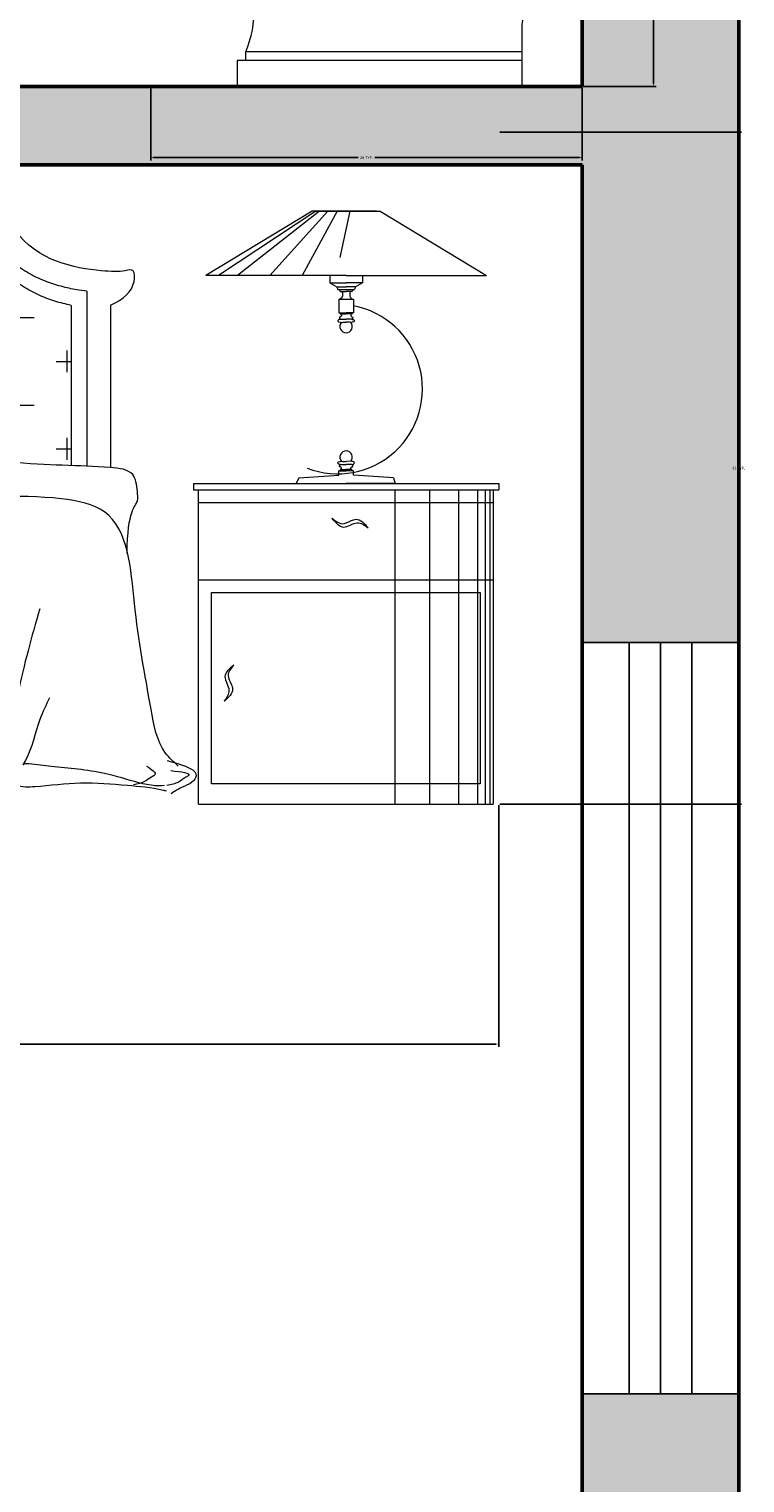
# Model space of a CAD drawing. Units: inches. Extents: x 1771 to 3025, y 319 to 889.
# Tile 5 of 35: x 2055 to 2101, y 527 to 620. Entities that reach past the tile are written whole.
import ezdxf

# ---------------------------------------------------------------- set-up
doc = ezdxf.new("R2010")
doc.units = ezdxf.units.IN
doc.header["$MEASUREMENT"] = 0
for name, color, linetype, lineweight in [('A-ANNO-DIMS', 2, 'Continuous', 18), ('A-FLOR-FIXT', 8, 'Continuous', 18), ('A-FURN', 8, 'Continuous', 18), ('A-GLAZ', 40, 'Continuous', 25), ('A-WALL', 7, 'Continuous', 50), ('A-WALL-PATT', 254, 'Continuous', 13)]:
    doc.layers.add(name, color=color, linetype=linetype, lineweight=lineweight)
doc.styles.get("Standard").update_dxf_attribs({"font": 'arial.ttf'})
doc.dimstyles.get("Standard").update_dxf_attribs({"dimtxt": 0.18, "dimasz": 0.18, "dimexe": 0.18, "dimexo": 0.0625, "dimgap": 0.09, "dimtad": 0, "dimtih": 1, "dimtoh": 1, "dimdec": 4, "dimzin": 0, "dimdsep": 46, "dimtxsty": 'Standard', "dimcen": 0.09, "dimadec": 0, "dimazin": 0, "dimtfac": 1, "dimtdec": 4, "dimtofl": 0, "dimtmove": 0, "dimatfit": 3, "dimfxl": 1, "dimtolj": 1, "dimtzin": 0, "dimarcsym": 0})

# ---------------------------------------------------------------- blocks, each defined once
blk = doc.blocks.new('A$C3908634B')
for p, q in [((2198.9, 923.4), (2033.5, 823.1)), ((2204.8, 923.4), (2053.3, 823.1)), ((2210.8, 923.4), (2082.7, 823.1)), ((2223.5, 923.4), (2133.1, 823.1)), ((2237.8, 923.4), (2183.8, 823.1)), ((2252, 923.4), (2198.9, 923.4)), ((2204.8, 923.4), (2252, 923.4)), ((2257.6, 923.4), (2242.2, 851.1)), ((2299.3, 923.4), (2252, 923.4)), ((2252, 923.4), (2305.2, 923.4)), ((2305.2, 923.4), (2470.5, 823.1)), ((2252, 823.1), (2033.5, 823.1)), ((2226.5, 823.1), (2226.5, 811.7)), ((2252, 823.1), (2470.5, 823.1)), ((2277.6, 823.1), (2277.6, 811.7)), ((1848.6, 798.8), (1848.6, 526.2)), ((2226.5, 811.7), (2237.6, 805.4)), ((2226.5, 811.7), (2252, 811.7)), ((2237.6, 805.4), (2239.1, 801.4)), ((2237.6, 805.4), (2252, 805.4)), ((2239.1, 801.4), (2264.9, 801.4)), ((2241.4, 801.4), (2242.8, 798.3)), ((2242.8, 798.3), (2245.8, 797.6)), ((2242.8, 798.3), (2252, 798.3)), ((2245.8, 797.6), (2246.5, 794.9)), ((2246.4, 793.9), (2246.1, 792.6)), ((2246.1, 792.6), (2246.1, 791.9)), ((2246.5, 794.9), (2246.4, 793.9)), ((2277.6, 811.7), (2252, 811.7)), ((2266.5, 805.4), (2252, 805.4)), ((2261.2, 798.3), (2252, 798.3)), ((2258.2, 797.6), (2257.6, 794.9)), ((2257.6, 794.9), (2257.6, 793.9)), ((2257.6, 793.9), (2257.9, 792.6)), ((2257.9, 792.6), (2258, 791.9)), ((2261.2, 798.3), (2258.2, 797.6)), ((2262.6, 801.4), (2261.2, 798.3)), ((2266.5, 805.4), (2264.9, 801.4)), ((2277.6, 811.7), (2266.5, 805.4)), ((1824, 776.5), (1824, 527.2)), ((2242.3, 786.4), (2240.7, 785.6)), ((2240.7, 785.6), (2240.7, 765)), ((2263.3, 785.6), (2240.7, 785.6)), ((2244.7, 788), (2242.3, 786.4)), ((2245.6, 790.5), (2244.7, 788)), ((2246.1, 791.1), (2245.6, 790.5)), ((2246.1, 791.9), (2246.1, 791.1)), ((2258, 791.9), (2258, 791.1)), ((2258, 791.1), (2258.4, 790.5)), ((2258.4, 790.5), (2259.4, 788)), ((2259.4, 788), (2261.7, 786.4)), ((2261.7, 786.4), (2263.3, 785.6)), ((2263.3, 785.6), (2263.3, 765)), ((1732.4, 757.6), (1766.5, 757.6)), ((2239.4, 753.5), (2239.2, 752.9)), ((2239.2, 752.9), (2239.3, 752.1)), ((2239.3, 752.1), (2239.7, 751.4)), ((2239.9, 753.9), (2239.4, 753.5)), ((2239.7, 751.4), (2240.2, 750.9)), ((2240.3, 754.3), (2239.9, 753.9)), ((2240.2, 750.9), (2242.6, 750.2)), ((2240.8, 754.6), (2240.3, 754.3)), ((2240.7, 765), (2242.1, 764.2)), ((2240.7, 765), (2252, 765)), ((2241.5, 754.7), (2240.8, 754.6)), ((2242.4, 754.7), (2241.5, 754.7)), ((2241.9, 757.9), (2241.7, 757.2)), ((2241.7, 757.2), (2241.8, 756.6)), ((2241.8, 756.6), (2242.3, 755.9)), ((2242.2, 758.5), (2241.9, 757.9)), ((2242.1, 764.2), (2243, 763.3)), ((2243.1, 758.7), (2242.2, 758.5)), ((2242.3, 755.9), (2243.4, 755.2)), ((2243.4, 755.2), (2242.4, 754.7)), ((2242.6, 750.2), (2244.4, 750)), ((2243, 763.3), (2243.9, 762.5)), ((2243, 763.3), (2252, 763.3)), ((2243.9, 759.1), (2243.1, 758.7)), ((2243.4, 755.2), (2252, 755.2)), ((2243.9, 762.5), (2244.6, 761.4)), ((2244.3, 759.5), (2243.9, 759.1)), ((2244.6, 760.2), (2244.3, 759.5)), ((2244.4, 750), (2246.9, 750.2)), ((2244.6, 761.4), (2244.6, 760.2)), ((2246.9, 750.2), (2252, 750.2)), ((2263.3, 765), (2252, 765)), ((2261.1, 763.3), (2252, 763.3)), ((2260.7, 755.2), (2252, 755.2)), ((2257.1, 750.2), (2252, 750.2)), ((2259.6, 750), (2257.1, 750.2)), ((2259.5, 761.4), (2259.4, 760.2)), ((2259.4, 760.2), (2259.7, 759.5)), ((2260.1, 762.5), (2259.5, 761.4)), ((2261.5, 750.2), (2259.6, 750)), ((2259.7, 759.5), (2260.1, 759.1)), ((2261.1, 763.3), (2260.1, 762.5)), ((2260.1, 759.1), (2260.9, 758.7)), ((2261.8, 755.9), (2260.7, 755.2)), ((2260.7, 755.2), (2261.6, 754.7)), ((2260.9, 758.7), (2261.8, 758.5)), ((2261.9, 764.2), (2261.1, 763.3)), ((2263.9, 750.9), (2261.5, 750.2)), ((2261.6, 754.7), (2262.5, 754.7)), ((2261.8, 758.5), (2262.2, 757.9)), ((2262.2, 756.6), (2261.8, 755.9)), ((2263.3, 765), (2261.9, 764.2)), ((2262.2, 757.9), (2262.4, 757.2)), ((2262.4, 757.2), (2262.2, 756.6)), ((2262.5, 754.7), (2263.2, 754.6)), ((2263.2, 754.6), (2263.8, 754.3)), ((2263.8, 754.3), (2264.2, 753.9)), ((2264.3, 751.4), (2263.9, 750.9)), ((2264.2, 753.9), (2264.7, 753.5)), ((2264.7, 752.1), (2264.3, 751.4)), ((2264.7, 753.5), (2264.8, 752.9)), ((2264.8, 752.9), (2264.7, 752.1)), ((1817.7, 672.4), (1817.7, 706.5)), ((1800.6, 689.4), (1824, 689.4)), ((1732.4, 621.3), (1766.5, 621.3)), ((1817.7, 536), (1817.7, 570.1)), ((1800.6, 553.1), (1824, 553.1)), ((2239.2, 530.9), (2239.3, 531.7)), ((2239.4, 530.3), (2239.2, 530.9)), ((2239.3, 531.7), (2239.7, 532.4)), ((2239.9, 529.9), (2239.4, 530.3)), ((2239.7, 532.4), (2240.2, 532.9)), ((2240.3, 529.5), (2239.9, 529.9)), ((2240.2, 532.9), (2242.6, 533.6)), ((2240.8, 529.2), (2240.3, 529.5)), ((2241.5, 529.1), (2240.8, 529.2)), ((2242.4, 529.1), (2241.5, 529.1)), ((2241.7, 526.6), (2241.8, 527.2)), ((2241.9, 525.9), (2241.7, 526.6)), ((2241.8, 527.2), (2242.3, 527.9)), ((2242.2, 525.3), (2241.9, 525.9)), ((2243.1, 525.1), (2242.2, 525.3)), ((2242.3, 527.9), (2243.4, 528.6)), ((2243.4, 528.6), (2242.4, 529.1)), ((2242.6, 533.6), (2244.4, 533.8)), ((2243, 520.5), (2243.9, 521.3)), ((2243.9, 524.7), (2243.1, 525.1)), ((2243.4, 528.6), (2252, 528.6)), ((2244.3, 524.3), (2243.9, 524.7)), ((2243.9, 521.3), (2244.6, 522.4)), ((2243.9, 521.3), (2252, 521.3)), ((2244.6, 523.6), (2244.3, 524.3)), ((2244.4, 533.8), (2246.9, 533.6)), ((2244.6, 522.4), (2244.6, 523.6)), ((2246.9, 533.6), (2252, 533.6)), ((2259.2, 533.8), (2252, 533.6)), ((2260.7, 528.6), (2252, 528.6)), ((2260.1, 521.3), (2252, 521.3)), ((2259.4, 523.6), (2259.7, 524.3)), ((2259.5, 522.4), (2259.4, 523.6)), ((2260.1, 521.3), (2259.5, 522.4)), ((2261.5, 533.6), (2259.6, 533.8)), ((2259.7, 524.3), (2260.1, 524.7)), ((2260.1, 524.7), (2260.9, 525.1)), ((2261.1, 520.5), (2260.1, 521.3)), ((2260.7, 528.6), (2261.6, 529.1)), ((2261.8, 527.9), (2260.7, 528.6)), ((2260.9, 525.1), (2261.8, 525.3)), ((2263.9, 532.9), (2261.5, 533.6)), ((2261.6, 529.1), (2262.5, 529.1)), ((2262.2, 527.2), (2261.8, 527.9)), ((2261.8, 525.3), (2262.2, 525.9)), ((2262.4, 526.6), (2262.2, 527.2)), ((2262.2, 525.9), (2262.4, 526.6)), ((2262.5, 529.1), (2263.2, 529.2)), ((2263.2, 529.2), (2263.8, 529.5)), ((2263.8, 529.5), (2264.2, 529.9)), ((2264.3, 532.4), (2263.9, 532.9)), ((2264.2, 529.9), (2264.7, 530.3)), ((2264.7, 531.7), (2264.3, 532.4)), ((2264.8, 530.9), (2264.7, 531.7)), ((2264.7, 530.3), (2264.8, 530.9)), ((2014.5, 499.5), (2489.5, 499.5)), ((2014.5, 499.5), (2014.5, 489.5)), ((2178.5, 507.9), (2174.2, 499.5)), ((2174.2, 499.5), (2252, 499.5)), ((2178.5, 507.9), (2240.7, 512.1)), ((2240.7, 518.8), (2242.1, 519.6)), ((2240.7, 512.1), (2240.7, 518.8)), ((2240.7, 518.8), (2252, 518.8)), ((2242.1, 519.6), (2243, 520.5)), ((2263.3, 518.8), (2252, 518.8)), ((2328.4, 499.5), (2252, 499.5)), ((2261.9, 519.6), (2261.1, 520.5)), ((2263.3, 518.8), (2261.9, 519.6)), ((2263.3, 512.1), (2263.3, 518.8)), ((2325.5, 507.9), (2263.3, 512.1)), ((2325.5, 507.9), (2328.4, 499.5)), ((2489.5, 499.5), (2489.5, 489.5)), ((2014.5, 489.5), (2489.5, 489.5)), ((2022.4, 0), (2022.4, 489.5)), ((2327.9, 488.6), (2327.9, 0)), ((2381.9, 488.6), (2381.9, 0)), ((2426.8, 488.6), (2426.8, 0)), ((2456.5, 488.6), (2456.5, 0)), ((2468.2, 488.6), (2468.2, 0)), ((2475.4, 488.6), (2475.4, 0)), ((2480.8, 489.5), (2480.8, 0)), ((2022.4, 469.5), (2480.8, 469.5)), ((2022.4, 349.5), (2480.8, 349.5)), ((2042.4, 329.5), (2460.8, 329.5)), ((2042.4, 31.6), (2042.4, 329.5)), ((2460.8, 329.5), (2460.8, 31.6)), ((2022.4, 281.6), (2022.4, 301.6)), ((2460.8, 31.6), (2042.4, 31.6)), ((2022.4, 0), (2480.8, 0))]:
    blk.add_line(p, q)
at = {"ltscale": 20}
blk.add_line((1885.4, 776.7), (1885.4, 524), dxfattribs=at)
for centre, radius, start, end in [((2239, 646.2), 131.8, 248.8, 79.3766), ((2252, 743.5), 9.69, 137.7341, 270), ((2252, 743.5), 9.69, 270, 42.2659), ((2252, 540.3), 9.69, 90, 222.2659), ((2252, 540.3), 9.69, 317.7341, 90)]:
    blk.add_arc(centre, radius, start, end)
blk.add_open_spline([(1885.4, 776.7), (1905.9, 786.2), (1923.9, 802.1), (1922.5, 834.8), (1905.3, 828.3), (1849.2, 830.4), (1763.4, 847.2), (1717.7, 924.2), (1691.7, 880.4), (1541.2, 907.1), (1472.8, 1014.1), (1283.8, 1035.5), (1218.1, 1046.3)], degree=3, knots=[12.417853, 12.417853, 12.417853, 12.417853, 68.394536, 90.665986, 114.156853, 157.554067, 281.869614, 298.858744, 338.737111, 347.060176, 470.423438, 625.498764, 625.498764, 625.498764, 625.498764], dxfattribs=at)
for points, knots in [([(1848.6, 798.8), (1836.4, 799.9), (1828.6, 801.3), (1812.5, 805), (1804.1, 807.2), (1787.2, 812.8), (1778.7, 816.1), (1761.8, 824.2), (1753.4, 828.9), (1738.5, 839), (1731.9, 844.1), (1721.5, 853.5), (1717.5, 857.5), (1713.7, 861.8)], [179.400376, 179.400376, 179.400376, 179.400376, 196.086144, 196.086144, 213.445516, 213.445516, 230.804888, 230.804888, 248.16426, 248.16426, 262.451931, 262.451931, 271.832526, 271.832526, 271.832526, 271.832526]), ([(1824, 776.5), (1822.9, 776.7), (1821.8, 777), (1812.5, 779.1), (1804.1, 781.3), (1787.2, 786.9), (1778.7, 790.3), (1761.8, 798.3), (1753.4, 803), (1738.5, 813.1), (1731.9, 818.2), (1721.5, 827.7), (1717.5, 831.7), (1713.7, 835.9)], [193.740688, 193.740688, 193.740688, 193.740688, 196.086144, 196.086144, 213.445516, 213.445516, 230.804888, 230.804888, 248.16426, 248.16426, 262.451931, 262.451931, 271.832526, 271.832526, 271.832526, 271.832526]), ([(2229.9, 445.5), (2235.6, 438.6), (2246.7, 424.9), (2268.5, 442.9), (2280.6, 434.4), (2286.1, 430.5)], [0, 0, 0, 0, 22.772447, 45.052082, 63.466582, 63.466582, 63.466582, 63.466582]), ([(2229.9, 445.5), (2235.2, 441.1), (2244.7, 433.2), (2257.6, 440.9), (2272.5, 446), (2280.3, 437.1), (2286.1, 430.5)], [0, 0, 0, 0, 18.381528, 32.980054, 40.875646, 63.595153, 63.595153, 63.595153, 63.595153]), ([(2077.2, 216.6), (2072.8, 211.4), (2064.9, 201.9), (2072.6, 189), (2077.8, 174.1), (2068.9, 166.3), (2062.3, 160.5)], [0, 0, 0, 0, 18.381528, 32.980054, 40.875646, 63.595153, 63.595153, 63.595153, 63.595153]), ([(2077.2, 216.6), (2070.3, 211), (2056.7, 199.9), (2074.6, 178.1), (2066.1, 166), (2062.3, 160.5)], [0, 0, 0, 0, 22.772447, 45.052082, 63.466582, 63.466582, 63.466582, 63.466582])]:
    blk.add_open_spline(points, degree=3, knots=knots)
at = {"ltscale": 5}
for points, knots in [([(1911, 390.4), (1911.9, 458.8), (1930, 464.8), (1926.5, 491.4), (1923.4, 520.4), (1870.5, 525.9), (1798, 527.2), (1556.5, 543.7), (1364.8, 538.4), (1259.7, 541.4)], [0, 0, 0, 0, 32.681627, 48.455722, 75.25348, 112.004017, 183.381957, 310.642358, 588.939547, 588.939547, 588.939547, 588.939547]), ([(1990.5, 59.4), (1983.5, 65.8), (1958.6, 88.6), (1942.6, 182.5), (1920.4, 297.5), (1912.1, 455.6), (1776.3, 485.5), (1526.4, 465.8), (1305.2, 468.9), (1210.9, 472.2)], [0, 0, 0, 0, 28.320233, 100.953775, 269.820348, 420.691469, 489.161544, 656.134073, 940.569207, 940.569207, 940.569207, 940.569207]), ([(1775.2, 304.1), (1762.7, 260.8), (1739, 178.1), (1727.3, 82.2), (1704.2, 38.3), (1700.3, 30.9)], [0, 0, 0, 0, 135.247847, 258.692787, 283.800228, 283.800228, 283.800228, 283.800228]), ([(1790.4, 165.6), (1785, 154.5), (1769.8, 123.2), (1763.1, 85), (1750.2, 63.5), (1748.7, 61.1)], [0, 0, 0, 0, 37.234018, 105.386078, 113.844905, 113.844905, 113.844905, 113.844905]), ([(1969.1, 28.9), (1964.3, 28.7), (1950.9, 28.3), (1919.6, 35.4), (1867.6, 52.4), (1808.2, 57), (1768, 61.4), (1751.8, 63.6), (1749.1, 61.4), (1748.7, 61.1)], [0, 0, 0, 0, 14.447875, 40.468341, 96.220884, 181.018327, 216.046098, 224.609189, 226.185962, 226.185962, 226.185962, 226.185962]), ([(1941.2, 59.4), (1949.3, 54.3), (1960, 47.4), (1946.7, 41.4), (1937.9, 33.4), (1927.5, 31.3), (1921, 30)], [0, 0, 0, 0, 19.035414, 25.269998, 36.960672, 56.00812, 56.00812, 56.00812, 56.00812]), ([(1979.3, 52.3), (1995.3, 50.6), (2014.9, 48.5), (1998.8, 40.1), (1989.9, 32.4), (1979.5, 30.2), (1973.1, 28.9)], [0, 0, 0, 0, 28.05485, 34.289435, 45.980108, 65.027556, 65.027556, 65.027556, 65.027556]), ([(1973.5, 67.9), (1979.4, 66.3), (1994.6, 62.3), (2025.5, 51), (2011.2, 31.6), (1995.7, 27.1), (1985.4, 20.1), (1979.9, 16.4)], [0, 0, 0, 0, 19.937155, 51.57724, 63.193909, 80.21631, 100.09061, 100.09061, 100.09061, 100.09061]), ([(1972.3, 20.4), (1970.7, 20.8), (1950, 25.9), (1906.5, 29.2), (1838.6, 35.6), (1782.4, 27.4), (1742.2, 25.9), (1729.1, 33.6), (1724.3, 36.5)], [590.079786, 590.079786, 590.079786, 590.079786, 594.646549, 651.888327, 725.747367, 797.841373, 826.274406, 843.189267, 843.189267, 843.189267, 843.189267])]:
    blk.add_open_spline(points, degree=3, knots=knots, dxfattribs=at)
blk = doc.blocks.new('A$C062C426B')
for p, q in [((0.4867, 0.6739, -0.3429), (0.4867, 0.6365, -0.3429)), ((0.4992, 0.6739, -0.3429), (0.4867, 0.6739, -0.3429)), ((0.5616, 0.6739, -0.3429), (0.5491, 0.6739, -0.3429)), ((0.5616, 0.6365, -0.3429), (0.5616, 0.6739, -0.3429)), ((0.4867, 0.6365, -0.3429), (0.4992, 0.6365, -0.3429)), ((0.4992, 0.6365, -0.3429), (0.4992, 0.577, -0.3429)), ((0.5491, 0.6365, -0.3429), (0.5616, 0.6365, -0.3429)), ((0.5491, 0.577, -0.3429), (0.5491, 0.6365, -0.3429)), ((0.624, 0.649, -0.3429), (0.599, 0.6365, -0.3429)), ((0.599, 0.6365, -0.3429), (0.599, 0.5616, -0.3429)), ((0.624, 0.5491, -0.3429), (0.624, 0.649, -0.3429)), ((0.599, 0.624, -0.3429), (0.5491, 0.624, -0.3429)), ((0.5521, 0.5741, -0.3429), (0.599, 0.5741, -0.3429)), ((0.599, 0.5616, -0.3429), (0.624, 0.5491, -0.3429)), ((0.4867, 0.5117, -0.3429), (0.5017, 0.5192, -0.3429)), ((0.4867, 0.4992, -0.3429), (0.4867, 0.5117, -0.3429)), ((0.5616, 0.5117, -0.3429), (0.5466, 0.5192, -0.3429)), ((0.5616, 0.4992, -0.3429), (0.5616, 0.5117, -0.3429)), ((0.4867, 0.4992, -0.3429), (0.4992, 0.4992, -0.3429)), ((0.4992, 0.4118, -0.3429), (0.4992, 0.4992, -0.3429)), ((0.5491, 0.4118, -0.3429), (0.5491, 0.4992, -0.3429)), ((0.5491, 0.4992, -0.3429), (0.5616, 0.4992, -0.3429)), ((0.4243, 0.4243, -0.3429), (0.0125, 0.4243, -0.3429)), ((0.0125, 0.4243, -0.3429), (0.0125, 0.3994, -0.3429)), ((0.4243, 0.3994, -0.3429), (0.4243, 0.4243, -0.3429)), ((0.4992, 0.4118, -0.3429), (0.4867, 0.4118, -0.3429)), ((0.4867, 0.4118, -0.3429), (0.4867, 0.3994, -0.3429)), ((0.5616, 0.4118, -0.3429), (0.5491, 0.4118, -0.3429)), ((0.5616, 0.3994, -0.3429), (0.5616, 0.4118, -0.3429)), ((0.5616, 0.3994, -0.3429), (0, 0.3994, -0.3429)), ((0, 0.3994, -0.3429), (0, 0.337, -0.3429)), ((0.5741, 0.3869, -0.3429), (0.5741, 0.1761, -0.3429)), ((0, 0.337, -0.3429), (0.4493, 0.337, -0.3429)), ((0.567, 0.1504, -0.3429), (0.5438, 0.1117, -0.3429)), ((0.5366, 0.086, -0.3429), (0.5366, 0, -0.3429)), ((0.5366, 0.0499, -0.3429), (0.1373, 0.0499, -0.3429)), ((0.1373, 0.0499, -0.3429), (0.1373, 0.0374, -0.3429)), ((0.5366, 0.0374, -0.3429), (0.1248, 0.0374, -0.3429)), ((0.1248, 0.0374, -0.3429), (0.1248, 0, -0.3429))]:
    blk.add_line(p, q)
for radius in [0.0374, 0.0125]:
    blk.add_circle((0.5242, 0.5491, -0.3429), radius)
for centre, radius, start, end in [((0.5242, 0.6552, -0.3429), 0.0312, 36.8699, 143.1301), ((0.5616, 0.3869, -0.3429), 0.0125, 0, 90), ((0.5429, 0.181, -0.3429), 0.1819, 95.9061, 120.9638), ((0.2791, 0.4017, -0.3429), 0.2664, 194.0552, 310.7015), ((-0.0044, 0.1107, -0.3429), 0.1542, 336.7818, 25.8778), ((0.5242, 0.1761, -0.3429), 0.0499, 329.0362, 0), ((0.5866, 0.086, -0.3429), 0.0499, 149.0362, 180)]:
    blk.add_arc(centre, radius, start, end)
blk = doc.blocks.new('WIN-48')
for p, q in [((0, 0), (0, 10)), ((48, 0), (48, 10)), ((0, 7), (48, 7)), ((0, 5), (48, 5)), ((0, 3), (48, 3))]:
    blk.add_line(p, q)
blk = doc.blocks.new('*D40')
at = {"layer": 'A-ANNO-DIMS', "color": 0, "lineweight": -2, "transparency": 16777216}
for p, q in [((1983.209, 570.711), (1983.209, 555.266)), ((2085.389, 570.711), (2085.389, 555.266)), ((1983.389, 555.446), (2033.223, 555.446)), ((2085.209, 555.446), (2035.375, 555.446))]:
    blk.add_line(p, q, dxfattribs=at)
at = {"layer": 'A-ANNO-DIMS', "color": 0, "transparency": 16777216}
for points in [[(1983.389, 555.476), (1983.389, 555.416), (1983.209, 555.446)], [(2085.209, 555.476), (2085.209, 555.416), (2085.389, 555.446)]]:
    blk.add_solid(points, dxfattribs=at)
at = {"layer": 'Defpoints', "color": 0, "transparency": 16777216}
for p in [(1983.209, 570.773), (2085.389, 570.773), (2085.389, 555.446)]:
    blk.add_point(p, dxfattribs=at)
at = {"layer": 'A-ANNO-DIMS', "color": 0, "transparency": 16777216, "insert": (2034.299, 555.446), "char_height": 0.18, "attachment_point": 5}
blk.add_mtext('\\A1;BED B2 102 TYP.', dxfattribs=at)
blk = doc.blocks.new('*D41')
at = {"layer": 'A-ANNO-DIMS', "color": 0, "lineweight": -2, "transparency": 16777216}
for p, q in [((2085.452, 613.716), (2100.896, 613.716)), ((2100.716, 613.536), (2100.716, 592.427)), ((2100.716, 570.953), (2100.716, 592.063)), ((2085.452, 570.773), (2100.896, 570.773))]:
    blk.add_line(p, q, dxfattribs=at)
at = {"layer": 'A-ANNO-DIMS', "color": 0, "transparency": 16777216}
for points in [[(2100.686, 613.536), (2100.746, 613.536), (2100.716, 613.716)], [(2100.686, 570.953), (2100.746, 570.953), (2100.716, 570.773)]]:
    blk.add_solid(points, dxfattribs=at)
at = {"layer": 'Defpoints', "color": 0, "transparency": 16777216}
for p in [(2085.389, 613.716), (2100.716, 613.716), (2085.389, 570.773)]:
    blk.add_point(p, dxfattribs=at)
at = {"layer": 'A-ANNO-DIMS', "color": 0, "transparency": 16777216, "insert": (2100.716, 592.245), "char_height": 0.18, "attachment_point": 5}
blk.add_mtext('\\A1;43 TYP.', dxfattribs=at)
blk = doc.blocks.new('*D52')
at = {"layer": 'A-ANNO-DIMS', "color": 0, "lineweight": -2, "transparency": 16777216}
for p, q in [((2090.786, 646.957), (2095.452, 646.957)), ((2095.272, 646.777), (2095.272, 631.979)), ((2095.272, 616.814), (2095.272, 631.612)), ((2090.786, 616.634), (2095.452, 616.634))]:
    blk.add_line(p, q, dxfattribs=at)
at = {"layer": 'A-ANNO-DIMS', "color": 0, "transparency": 16777216}
for points in [[(2095.242, 646.777), (2095.302, 646.777), (2095.272, 646.957)], [(2095.242, 616.814), (2095.302, 616.814), (2095.272, 616.634)]]:
    blk.add_solid(points, dxfattribs=at)
at = {"layer": 'Defpoints', "color": 0, "transparency": 16777216}
for p in [(2090.724, 646.957), (2095.272, 646.957), (2090.724, 616.634)]:
    blk.add_point(p, dxfattribs=at)
at = {"layer": 'A-ANNO-DIMS', "color": 0, "transparency": 16777216, "insert": (2095.272, 631.795), "char_height": 0.18, "attachment_point": 5}
blk.add_mtext('\\A1;WC 30 TYP.', dxfattribs=at)
blk = doc.blocks.new('*D53')
at = {"layer": 'A-ANNO-DIMS', "color": 0, "lineweight": -2, "transparency": 16777216}
for p, q in [((2063.157, 616.571), (2063.157, 611.905)), ((2090.724, 616.571), (2090.724, 611.905)), ((2063.337, 612.085), (2076.411, 612.085)), ((2090.544, 612.085), (2077.47, 612.085))]:
    blk.add_line(p, q, dxfattribs=at)
at = {"layer": 'A-ANNO-DIMS', "color": 0, "transparency": 16777216}
for points in [[(2063.337, 612.115), (2063.337, 612.055), (2063.157, 612.085)], [(2090.544, 612.115), (2090.544, 612.055), (2090.724, 612.085)]]:
    blk.add_solid(points, dxfattribs=at)
at = {"layer": 'Defpoints', "color": 0, "transparency": 16777216}
for p in [(2063.157, 616.634), (2090.724, 616.634), (2090.724, 612.085)]:
    blk.add_point(p, dxfattribs=at)
at = {"layer": 'A-ANNO-DIMS', "color": 0, "transparency": 16777216, "insert": (2076.94, 612.085), "char_height": 0.18, "attachment_point": 5}
blk.add_mtext('\\A1;28 TYP.', dxfattribs=at)

msp = doc.modelspace()

# ---------------------------------------------------------------- hatches: boundary and pattern name
at = {"layer": 'A-WALL-PATT'}
h = msp.add_hatch(color=256, dxfattribs=at)
h.dxf.hatch_style = 1
h.paths.add_polyline_path([(1870.724, 888.634), (1799.724, 888.634), (1799.724, 878.634), (1870.724, 878.634)])
h.paths.add_polyline_path([(1968.767, 888.634), (1918.724, 888.634), (1918.724, 878.634), (1941.724, 878.634), (1941.724, 830.634), (1946.724, 830.634), (1946.724, 878.634), (1968.767, 878.634)])
h.paths.add_polyline_path([(2059.676, 888.634), (2016.767, 888.634), (2016.767, 878.634), (2037.724, 878.634), (2037.724, 794.634), (1941.724, 794.634), (1941.724, 758.634), (1941.724, 664.634), (1946.724, 664.634), (1946.724, 712), (1946.724, 789.634), (2054.724, 789.634), (2054.724, 794.634), (2042.325, 794.634), (2042.325, 798.62), (2042.325, 835.497), (2042.724, 878.634), (2059.676, 878.634)])
h.paths.add_polyline_path([(2100.724, 888.634), (2077.676, 888.634), (2077.676, 878.634), (2090.724, 878.634), (2090.724, 789.634), (2090.724, 768.608), (2100.724, 768.608)])
h.paths.add_polyline_path([(2100.724, 720.608), (2090.724, 720.608), (2090.724, 669.634), (1982.724, 669.634), (1982.724, 664.634), (2001.724, 664.634), (2001.724, 652.634), (2006.724, 652.634), (2006.724, 664.634), (2049.518, 664.634, -0.385549), (2050.522, 664.634), (2090.724, 664.634), (2090.724, 649.173), (2100.724, 649.173)])
edge = h.paths.add_edge_path()
edge.add_line((2100.724, 631.173), (2090.724, 631.173))
edge.add_line((2090.724, 631.173), (2090.724, 616.634))
edge.add_line((2090.724, 616.634), (2001.724, 616.634))
edge.add_line((2001.724, 616.634), (1982.724, 616.634))
edge.add_line((1982.724, 616.634), (1982.724, 611.634))
edge.add_line((1982.724, 611.634), (2024.672, 611.634))
edge.add_spline(control_points=[(2024.672, 611.634), (2027.581, 612.871), (2030.014, 613.313), (2032.469, 613.716)], knot_values=[484.321569, 484.321569, 484.321569, 484.321569, 625.498764, 625.498764, 625.498764, 625.498764], degree=3, periodic=0)
edge.add_line((2032.469, 613.716), (2033.205, 613.716))
edge.add_spline(control_points=[(2033.205, 613.716), (2035.66, 613.313), (2039.461, 612.871), (2042.204, 611.634)], knot_values=[484.321569, 484.321569, 484.321569, 484.321569, 625.498764, 625.498764, 625.498764, 625.498764], degree=3, periodic=0)
edge.add_line((2042.204, 611.634), (2090.724, 611.634))
edge.add_line((2090.724, 611.634), (2090.724, 581.106))
edge.add_line((2090.724, 581.106), (2100.724, 581.106))
edge.add_line((2100.724, 581.106), (2100.724, 631.173))
h.paths.add_polyline_path([(2100.724, 533.106), (2090.724, 533.106), (2090.724, 479.634), (1946.724, 479.634), (1946.724, 616.634), (1936.724, 616.634), (1936.724, 543.634), (1845.724, 543.634), (1845.724, 533.634), (1936.724, 533.634), (1936.724, 469.634), (2090.724, 469.634), (2090.724, 452.762), (2100.724, 452.762)])
h.paths.add_polyline_path([(2100.724, 404.762), (2090.724, 404.762), (2090.724, 393.634), (1936.724, 393.634), (1936.724, 383.634), (2100.724, 383.634)])
h.paths.add_polyline_path([(1905.724, 758.634), (1835.47, 758.634), (1835.47, 758.634), (1813.444, 758.634), (1809.724, 758.634), (1809.724, 842.589, -0.008336), (1808.421, 842.634), (1799.724, 842.634), (1799.724, 690.584), (1809.724, 690.584), (1809.724, 753.634), (1905.724, 753.634)])
h.paths.add_polyline_path([(1809.724, 642.584), (1799.724, 642.584), (1799.724, 533.634), (1809.724, 533.634), (1809.724, 581)])

# ---------------------------------------------------------------- linework, layer by layer
at = {"layer": 'A-WALL'}
for p, q in [((2100.724, 383.634), (2100.724, 888.432)), ((2090.724, 616.634), (2090.724, 664.634)), ((2090.724, 616.634), (2001.724, 616.634)), ((2090.724, 611.634), (1982.724, 611.634)), ((2090.724, 479.634), (2090.724, 611.634))]:
    msp.add_line(p, q, dxfattribs=at)

# ---------------------------------------------------------------- block references
at = {"layer": 'A-FLOR-FIXT', "xscale": 44.17762020618112, "yscale": 44.17762020618112, "zscale": 44.17762020618112}
msp.add_blockref('A$C062C426B', (2063.157, 616.634, 15.147), dxfattribs=at)
at = {"layer": 'A-FURN', "xscale": 0.0410441893854556, "yscale": 0.0410441893854556, "zscale": 0.0410441893854556}
msp.add_blockref('A$C3908634B', (1983.209, 570.773), dxfattribs=at)
at = {"layer": 'A-GLAZ', "rotation": 270.0000000000006}
msp.add_blockref('WIN-48', (2090.724, 581.106), dxfattribs=at)

# ---------------------------------------------------------------- dimensions: what is measured, and where the dimension line sits
at = {"layer": 'A-ANNO-DIMS'}
for base, p1, p2, text, picture, middle in [((2095.272, 646.957), (2090.724, 616.634), (2090.724, 646.957), 'WC <> TYP.', '*D52', (2095.272, 631.795)), ((2100.716, 613.716), (2085.389, 570.773), (2085.389, 613.716), '<> TYP.', '*D41', (2100.716, 592.245))]:
    dim = msp.add_linear_dim(base=base, p1=p1, p2=p2, angle=90, text=text, dimstyle='Standard', override={"dimdec": 0, "dimrnd": 0, "dimzin": 0, "dimlunit": 2}, dxfattribs=at)
    dim.commit()
    dim.dimension.update_dxf_attribs({"geometry": picture, "text_midpoint": middle})
for base, p1, p2, text, picture, middle in [((2090.724, 612.085), (2063.157, 616.634), (2090.724, 616.634), '<> TYP.', '*D53', (2076.94, 612.085)), ((2085.389, 555.446), (1983.209, 570.773), (2085.389, 570.773), 'BED B2 <> TYP.', '*D40', (2034.299, 555.446))]:
    dim = msp.add_linear_dim(base=base, p1=p1, p2=p2, text=text, dimstyle='Standard', override={"dimdec": 0, "dimrnd": 0, "dimzin": 0, "dimlunit": 2}, dxfattribs=at)
    dim.commit()
    dim.dimension.update_dxf_attribs({"geometry": picture, "text_midpoint": middle})

doc.saveas('drawing.dxf')
